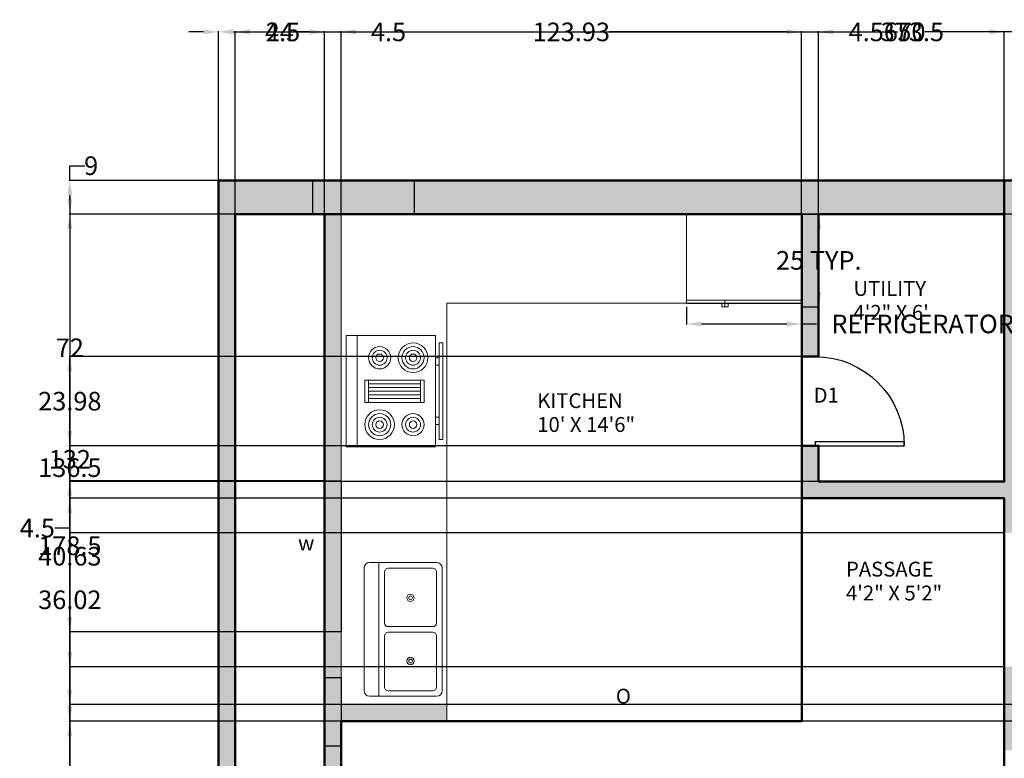
# Model space of a CAD drawing. Units: inches. Extents: x -12 to 887, y 330 to 874.
# Tile 3 of 9: x -12 to 253, y 675 to 874. Entities that reach past the tile are written whole.
import ezdxf

# ---------------------------------------------------------------- set-up
doc = ezdxf.new("R2010")
doc.units = ezdxf.units.IN
doc.header["$MEASUREMENT"] = 0
for name, color, linetype, lineweight in [('A-ANNO-DIMS', 2, 'Continuous', 18), ('A-ANNO-TEXT', 3, 'Continuous', 18), ('A-AREA-IDEN', 7, 'Continuous', 18), ('A-DOOR', 4, 'Continuous', 25), ('A-EQPM', 8, 'Continuous', 18), ('A-FLOR-FIXT', 8, 'Continuous', 18), ('A-GLAZ', 4, 'Continuous', 25), ('A-WALL', 7, 'Continuous', 50), ('A-WALL-PATT', 5, 'Continuous', 13)]:
    doc.layers.add(name, color=color, linetype=linetype, lineweight=lineweight)
doc.styles.get("Standard").update_dxf_attribs({"font": 'arial.ttf'})
doc.dimstyles.get("Standard").update_dxf_attribs({"dimtxt": 5, "dimasz": 4, "dimexe": 0.18, "dimexo": 0.0625, "dimgap": 0.09, "dimtad": 0, "dimtih": 1, "dimtoh": 1, "dimdec": 1, "dimzin": 0, "dimdsep": 46, "dimlunit": 4, "dimtxsty": 'Standard', "dimcen": 0.09, "dimadec": 0, "dimazin": 0, "dimtfac": 1, "dimtdec": 1, "dimtofl": 0, "dimtmove": 0, "dimatfit": 3, "dimfxl": 1, "dimtolj": 1, "dimtzin": 0, "dimarcsym": 0})

# ---------------------------------------------------------------- blocks, each defined once
blk = doc.blocks.new('Sink-double - 36 in top')
for p, q in [((-18, -4), (18, -4)), ((-0.75, -18.5), (-0.75, -6.5)), ((0.75, -6.5), (0.75, -18.5))]:
    blk.add_line(p, q)
for points in [[(-16.5, 0), (16.5, 0)], [(-18, -19.5), (-18, -1.5)], [(18, -1.5), (18, -19.5)], [(-16.5, -18.5), (-16.5, -6.5)], [(-15.5, -5.5), (-1.75, -5.5)], [(1.75, -5.5), (15.5, -5.5)], [(16.5, -6.5), (16.5, -18.5)], [(16.5, -21), (-16.5, -21)], [(-1.75, -19.5), (-15.5, -19.5)], [(15.5, -19.5), (1.75, -19.5)]]:
    blk.add_lwpolyline(points)
for centre, radius in [((-8.5, -12.5), 1), ((-8.5, -12.5), 0.5), ((8.5, -12.5), 1), ((8.5, -12.5), 0.5)]:
    blk.add_circle(centre, radius)
for centre, radius, start, end in [((-16.5, -1.5), 1.5, 90, 180), ((16.5, -1.5), 1.5, 0, 90), ((-15.5, -6.5), 1, 90, 180), ((-1.75, -6.5), 1, 0, 90), ((1.75, -6.5), 1, 90, 180), ((15.5, -6.5), 1, 0, 90), ((-15.5, -18.5), 1, 180, 270), ((-1.75, -18.5), 1, 270, 0), ((1.75, -18.5), 1, 180, 270), ((15.5, -18.5), 1, 270, 0), ((-16.5, -19.5), 1.5, 180, 270), ((16.5, -19.5), 1.5, 270, 0)]:
    blk.add_arc(centre, radius, start, end)
blk = doc.blocks.new('Range-Oven - 30 in top')
for p, q in [((0, -3), (30, -3)), ((12, -6), (18, -6)), ((13, -20), (13, -6)), ((14, -6), (14, -20)), ((15, -20), (15, -6)), ((16, -6), (16, -20)), ((17, -20), (17, -6)), ((18, -20), (12, -20)), ((6, -24), (6, -25)), ((8, -25), (8, -24)), ((22, -25), (22, -24)), ((24, -24), (24, -25))]:
    blk.add_line(p, q)
for points in [[(0, -24), (0, 0), (30, 0), (30, -24)], [(12, -21), (12, -5), (18, -5), (18, -21)], [(2, -26), (2, -25), (28, -25), (28, -26)]]:
    blk.add_lwpolyline(points, close=True)
for centre, radius in [((6, -9), 4), ((6, -9), 3), ((6, -9), 2), ((24, -9), 3), ((24, -9), 2), ((6, -9), 1), ((24, -9), 1), ((6, -18), 3), ((24, -18), 4), ((24, -18), 3), ((6, -18), 2), ((6, -18), 1), ((24, -18), 2), ((24, -18), 1)]:
    blk.add_circle(centre, radius)
blk = doc.blocks.new('Refrigerator-2 door - 36 in top')
for p, q in [((0, -26.999999), (36, -26.999999)), ((12, -26.999999), (12, -28.999999)), ((11, -27.999999), (11, -28.999999)), ((11, -28.999999), (13, -28.999999)), ((13, -28.999999), (13, -27.999999))]:
    blk.add_line(p, q)
blk.add_lwpolyline([(0, -27.999999), (0, 0), (36, 0), (36, -27.999999)], close=True)
blk = doc.blocks.new('*U5')
for p, q in [((0, 0), (0, -6)), ((40, 0), (40, -6))]:
    blk.add_line(p, q)
blk.add_lwpolyline([(0, 0), (0, 40), (1.75, 40), (1.75, 0)], close=True)
blk.add_arc((0, 0), 40, 0, 90)
blk = doc.blocks.new('*D28')
at = {"layer": 'A-ANNO-DIMS', "color": 0, "lineweight": -2, "transparency": 16777216}
for p, q in [((167.93, 796.66), (167.93, 791.9)), ((198.86, 796.66), (198.86, 791.9)), ((171.93, 792.08), (194.86, 792.08)), ((198.86, 792.08), (202.86, 792.08))]:
    blk.add_line(p, q, dxfattribs=at)
at = {"layer": 'A-ANNO-DIMS', "color": 0, "transparency": 16777216}
for points in [[(171.93, 792.75), (171.93, 791.42), (167.93, 792.08)], [(194.86, 792.75), (194.86, 791.42), (198.86, 792.08)]]:
    blk.add_solid(points, dxfattribs=at)
at = {"layer": 'Defpoints', "color": 0, "transparency": 16777216}
for p in [(167.93, 796.72), (198.86, 796.72), (198.86, 792.08)]:
    blk.add_point(p, dxfattribs=at)
at = {"layer": 'A-ANNO-DIMS', "color": 0, "transparency": 16777216, "insert": (243.71, 792.08), "char_height": 5, "attachment_point": 5}
blk.add_mtext('\\A1;REFRIGERATOR 31 TYP.', dxfattribs=at)
blk = doc.blocks.new('*D29')
at = {"layer": 'A-ANNO-DIMS', "color": 0, "lineweight": -2, "transparency": 16777216}
for p, q in [((198.92, 821.64), (203.68, 821.64)), ((203.5, 817.64), (203.5, 811.82)), ((203.5, 800.72), (203.5, 806.54)), ((198.92, 796.72), (203.68, 796.72))]:
    blk.add_line(p, q, dxfattribs=at)
at = {"layer": 'A-ANNO-DIMS', "color": 0, "transparency": 16777216}
for points in [[(202.83, 817.64), (204.17, 817.64), (203.5, 821.64)], [(202.83, 800.72), (204.17, 800.72), (203.5, 796.72)]]:
    blk.add_solid(points, dxfattribs=at)
at = {"layer": 'Defpoints', "color": 0, "transparency": 16777216}
for p in [(198.86, 821.64), (203.5, 821.64), (198.86, 796.72)]:
    blk.add_point(p, dxfattribs=at)
at = {"layer": 'A-ANNO-DIMS', "color": 0, "transparency": 16777216, "insert": (203.5, 809.18), "char_height": 5, "attachment_point": 5}
blk.add_mtext('\\A1;25 TYP.', dxfattribs=at)
blk = doc.blocks.new('*D38')
at = {"layer": 'A-ANNO-DIMS', "color": 0, "lineweight": -2, "transparency": 16777216}
for p, q in [((41.93, 830.72), (41.93, 870.84)), ((45.93, 870.66), (220.13, 870.66)), ((411.43, 870.66), (237.22, 870.66)), ((415.43, 830.72), (415.43, 870.84))]:
    blk.add_line(p, q, dxfattribs=at)
at = {"layer": 'A-ANNO-DIMS', "color": 0, "transparency": 16777216}
for points in [[(45.93, 871.33), (45.93, 869.99), (41.93, 870.66)], [(411.43, 871.33), (411.43, 869.99), (415.43, 870.66)]]:
    blk.add_solid(points, dxfattribs=at)
at = {"layer": 'Defpoints', "color": 0, "transparency": 16777216}
for p in [(415.43, 870.66), (41.93, 830.66), (415.43, 830.66)]:
    blk.add_point(p, dxfattribs=at)
at = {"layer": 'A-ANNO-DIMS', "color": 0, "transparency": 16777216, "insert": (228.68, 870.66), "char_height": 5, "attachment_point": 5}
blk.add_mtext('\\A1;373.5', dxfattribs=at)
blk = doc.blocks.new('*D39')
at = {"layer": 'A-ANNO-DIMS', "color": 0, "lineweight": -2, "transparency": 16777216}
for p, q in [((37.93, 870.66), (33.93, 870.66)), ((41.93, 830.72), (41.93, 870.84)), ((46.43, 821.72), (46.43, 870.84)), ((50.43, 870.66), (54.43, 870.66))]:
    blk.add_line(p, q, dxfattribs=at)
at = {"layer": 'A-ANNO-DIMS', "color": 0, "transparency": 16777216}
for points in [[(37.93, 871.33), (37.93, 869.99), (41.93, 870.66)], [(50.43, 871.33), (50.43, 869.99), (46.43, 870.66)]]:
    blk.add_solid(points, dxfattribs=at)
at = {"layer": 'Defpoints', "color": 0, "transparency": 16777216}
for p in [(46.43, 870.66), (41.93, 830.66), (46.43, 821.66)]:
    blk.add_point(p, dxfattribs=at)
at = {"layer": 'A-ANNO-DIMS', "color": 0, "transparency": 16777216, "insert": (59.19, 870.66), "char_height": 5, "attachment_point": 5}
blk.add_mtext('\\A1;4.5', dxfattribs=at)
blk = doc.blocks.new('*D40')
at = {"layer": 'A-ANNO-DIMS', "color": 0, "lineweight": -2, "transparency": 16777216}
for p, q in [((46.43, 821.72), (46.43, 870.84)), ((50.43, 870.66), (54.72, 870.66)), ((66.43, 870.66), (62.13, 870.66)), ((70.43, 821.72), (70.43, 870.84))]:
    blk.add_line(p, q, dxfattribs=at)
at = {"layer": 'A-ANNO-DIMS', "color": 0, "transparency": 16777216}
for points in [[(50.43, 871.33), (50.43, 869.99), (46.43, 870.66)], [(66.43, 871.33), (66.43, 869.99), (70.43, 870.66)]]:
    blk.add_solid(points, dxfattribs=at)
at = {"layer": 'Defpoints', "color": 0, "transparency": 16777216}
for p in [(70.43, 870.66), (46.43, 821.66), (70.43, 821.66)]:
    blk.add_point(p, dxfattribs=at)
at = {"layer": 'A-ANNO-DIMS', "color": 0, "transparency": 16777216, "insert": (58.43, 870.66), "char_height": 5, "attachment_point": 5}
blk.add_mtext('\\A1;24', dxfattribs=at)
blk = doc.blocks.new('*D41')
at = {"layer": 'A-ANNO-DIMS', "color": 0, "lineweight": -2, "transparency": 16777216}
for p, q in [((66.43, 870.66), (62.43, 870.66)), ((70.43, 821.72), (70.43, 870.84)), ((74.93, 821.72), (74.93, 870.84)), ((78.93, 870.66), (82.93, 870.66))]:
    blk.add_line(p, q, dxfattribs=at)
at = {"layer": 'A-ANNO-DIMS', "color": 0, "transparency": 16777216}
for points in [[(66.43, 871.33), (66.43, 869.99), (70.43, 870.66)], [(78.93, 871.33), (78.93, 869.99), (74.93, 870.66)]]:
    blk.add_solid(points, dxfattribs=at)
at = {"layer": 'Defpoints', "color": 0, "transparency": 16777216}
for p in [(74.93, 870.66), (70.43, 821.66), (74.93, 821.66)]:
    blk.add_point(p, dxfattribs=at)
at = {"layer": 'A-ANNO-DIMS', "color": 0, "transparency": 16777216, "insert": (87.69, 870.66), "char_height": 5, "attachment_point": 5}
blk.add_mtext('\\A1;4.5', dxfattribs=at)
blk = doc.blocks.new('*D42')
at = {"layer": 'A-ANNO-DIMS', "color": 0, "lineweight": -2, "transparency": 16777216}
for p, q in [((74.93, 821.72), (74.93, 870.84)), ((78.93, 870.66), (126.66, 870.66)), ((194.86, 870.66), (147.13, 870.66)), ((198.86, 821.7), (198.86, 870.84))]:
    blk.add_line(p, q, dxfattribs=at)
at = {"layer": 'A-ANNO-DIMS', "color": 0, "transparency": 16777216}
for points in [[(78.93, 871.33), (78.93, 869.99), (74.93, 870.66)], [(194.86, 871.33), (194.86, 869.99), (198.86, 870.66)]]:
    blk.add_solid(points, dxfattribs=at)
at = {"layer": 'Defpoints', "color": 0, "transparency": 16777216}
for p in [(198.86, 870.66), (74.93, 821.66), (198.86, 821.64)]:
    blk.add_point(p, dxfattribs=at)
at = {"layer": 'A-ANNO-DIMS', "color": 0, "transparency": 16777216, "insert": (136.89, 870.66), "char_height": 5, "attachment_point": 5}
blk.add_mtext('\\A1;123.93', dxfattribs=at)
blk = doc.blocks.new('*D43')
at = {"layer": 'A-ANNO-DIMS', "color": 0, "lineweight": -2, "transparency": 16777216}
for p, q in [((194.86, 870.66), (190.86, 870.66)), ((198.86, 821.7), (198.86, 870.84)), ((203.43, 821.72), (203.43, 870.84)), ((207.43, 870.66), (211.43, 870.66))]:
    blk.add_line(p, q, dxfattribs=at)
at = {"layer": 'A-ANNO-DIMS', "color": 0, "transparency": 16777216}
for points in [[(194.86, 871.33), (194.86, 869.99), (198.86, 870.66)], [(207.43, 871.33), (207.43, 869.99), (203.43, 870.66)]]:
    blk.add_solid(points, dxfattribs=at)
at = {"layer": 'Defpoints', "color": 0, "transparency": 16777216}
for p in [(203.43, 870.66), (198.86, 821.64), (203.43, 821.66)]:
    blk.add_point(p, dxfattribs=at)
at = {"layer": 'A-ANNO-DIMS', "color": 0, "transparency": 16777216, "insert": (220.05, 870.66), "char_height": 5, "attachment_point": 5}
blk.add_mtext('\\A1;4.567', dxfattribs=at)
blk = doc.blocks.new('*D44')
at = {"layer": 'A-ANNO-DIMS', "color": 0, "lineweight": -2, "transparency": 16777216}
for p, q in [((203.43, 821.72), (203.43, 870.84)), ((207.43, 870.66), (224.76, 870.66)), ((249.43, 870.66), (232.09, 870.66)), ((253.43, 821.72), (253.43, 870.84))]:
    blk.add_line(p, q, dxfattribs=at)
at = {"layer": 'A-ANNO-DIMS', "color": 0, "transparency": 16777216}
for points in [[(207.43, 871.33), (207.43, 869.99), (203.43, 870.66)], [(249.43, 871.33), (249.43, 869.99), (253.43, 870.66)]]:
    blk.add_solid(points, dxfattribs=at)
at = {"layer": 'Defpoints', "color": 0, "transparency": 16777216}
for p in [(253.43, 870.66), (203.43, 821.66), (253.43, 821.66)]:
    blk.add_point(p, dxfattribs=at)
at = {"layer": 'A-ANNO-DIMS', "color": 0, "transparency": 16777216, "insert": (228.43, 870.66), "char_height": 5, "attachment_point": 5}
blk.add_mtext('\\A1;50', dxfattribs=at)
blk = doc.blocks.new('*D45')
at = {"layer": 'A-ANNO-DIMS', "color": 0, "lineweight": -2, "transparency": 16777216}
for p, q in [((249.43, 870.66), (245.43, 870.66)), ((253.43, 821.72), (253.43, 870.84)), ((257.93, 821.72), (257.93, 870.84)), ((261.93, 870.66), (265.93, 870.66))]:
    blk.add_line(p, q, dxfattribs=at)
at = {"layer": 'A-ANNO-DIMS', "color": 0, "transparency": 16777216}
for points in [[(249.43, 871.33), (249.43, 869.99), (253.43, 870.66)], [(261.93, 871.33), (261.93, 869.99), (257.93, 870.66)]]:
    blk.add_solid(points, dxfattribs=at)
at = {"layer": 'Defpoints', "color": 0, "transparency": 16777216}
for p in [(257.93, 870.66), (253.43, 821.66), (257.93, 821.66)]:
    blk.add_point(p, dxfattribs=at)
at = {"layer": 'A-ANNO-DIMS', "color": 0, "transparency": 16777216, "insert": (270.69, 870.66), "char_height": 5, "attachment_point": 5}
blk.add_mtext('\\A1;4.5', dxfattribs=at)
blk = doc.blocks.new('*D53')
at = {"layer": 'A-ANNO-DIMS', "color": 0, "lineweight": -2, "transparency": 16777216}
for p, q in [((41.86, 830.66), (1.75, 830.66)), ((1.93, 826.66), (1.93, 604.54)), ((1.93, 377.16), (1.93, 599.28)), ((41.86, 373.16), (1.75, 373.16))]:
    blk.add_line(p, q, dxfattribs=at)
at = {"layer": 'A-ANNO-DIMS', "color": 0, "transparency": 16777216}
for points in [[(1.26, 826.66), (2.59, 826.66), (1.93, 830.66)], [(1.26, 377.16), (2.59, 377.16), (1.93, 373.16)]]:
    blk.add_solid(points, dxfattribs=at)
at = {"layer": 'Defpoints', "color": 0, "transparency": 16777216}
for p in [(1.93, 830.66), (41.93, 830.66), (41.93, 373.16)]:
    blk.add_point(p, dxfattribs=at)
at = {"layer": 'A-ANNO-DIMS', "color": 0, "transparency": 16777216, "insert": (1.93, 601.91), "char_height": 5, "attachment_point": 5}
blk.add_mtext('\\A1;457.5', dxfattribs=at)
blk = doc.blocks.new('*D57')
at = {"layer": 'A-ANNO-DIMS', "color": 0, "lineweight": -2, "transparency": 16777216}
for p, q in [((74.86, 685.16), (1.75, 685.16)), ((1.93, 681.16), (1.93, 628.55)), ((1.93, 570.66), (1.93, 623.27)), ((74.86, 566.66), (1.75, 566.66))]:
    blk.add_line(p, q, dxfattribs=at)
at = {"layer": 'A-ANNO-DIMS', "color": 0, "transparency": 16777216}
for points in [[(1.26, 681.16), (2.59, 681.16), (1.93, 685.16)], [(1.26, 570.66), (2.59, 570.66), (1.93, 566.66)]]:
    blk.add_solid(points, dxfattribs=at)
at = {"layer": 'Defpoints', "color": 0, "transparency": 16777216}
for p in [(1.93, 685.16), (74.93, 685.16), (74.93, 566.66)]:
    blk.add_point(p, dxfattribs=at)
at = {"layer": 'A-ANNO-DIMS', "color": 0, "transparency": 16777216, "insert": (1.93, 625.91), "char_height": 5, "attachment_point": 5}
blk.add_mtext('\\A1;118.5', dxfattribs=at)
blk = doc.blocks.new('*D58')
at = {"layer": 'A-ANNO-DIMS', "color": 0, "lineweight": -2, "transparency": 16777216}
for p, q in [((74.86, 821.66), (1.75, 821.66)), ((1.93, 817.66), (1.93, 756.06)), ((1.93, 689.16), (1.93, 750.77)), ((74.86, 685.16), (1.75, 685.16))]:
    blk.add_line(p, q, dxfattribs=at)
at = {"layer": 'A-ANNO-DIMS', "color": 0, "transparency": 16777216}
for points in [[(1.26, 817.66), (2.59, 817.66), (1.93, 821.66)], [(1.26, 689.16), (2.59, 689.16), (1.93, 685.16)]]:
    blk.add_solid(points, dxfattribs=at)
at = {"layer": 'Defpoints', "color": 0, "transparency": 16777216}
for p in [(1.93, 821.66), (74.93, 821.66), (74.93, 685.16)]:
    blk.add_point(p, dxfattribs=at)
at = {"layer": 'A-ANNO-DIMS', "color": 0, "transparency": 16777216, "insert": (1.93, 753.41), "char_height": 5, "attachment_point": 5}
blk.add_mtext('\\A1;136.5', dxfattribs=at)
blk = doc.blocks.new('*D59')
at = {"layer": 'A-ANNO-DIMS', "color": 0, "lineweight": -2, "transparency": 16777216}
for p, q in [((1.93, 830.66), (1.93, 834.66)), ((1.93, 834.66), (5.93, 834.66)), ((41.86, 830.66), (1.75, 830.66)), ((1.93, 825.66), (1.93, 826.66)), ((74.86, 821.66), (1.75, 821.66))]:
    blk.add_line(p, q, dxfattribs=at)
at = {"layer": 'A-ANNO-DIMS', "color": 0, "transparency": 16777216}
for points in [[(1.26, 826.66), (2.59, 826.66), (1.93, 830.66)], [(1.26, 825.66), (2.59, 825.66), (1.93, 821.66)]]:
    blk.add_solid(points, dxfattribs=at)
at = {"layer": 'Defpoints', "color": 0, "transparency": 16777216}
for p in [(1.93, 830.66), (41.93, 830.66), (74.93, 821.66)]:
    blk.add_point(p, dxfattribs=at)
at = {"layer": 'A-ANNO-DIMS', "color": 0, "transparency": 16777216, "insert": (7.66, 834.66), "char_height": 5, "attachment_point": 5}
blk.add_mtext('\\A1;9', dxfattribs=at)
blk = doc.blocks.new('*D69')
at = {"layer": 'A-ANNO-DIMS', "color": 0, "lineweight": -2, "transparency": 16777216}
for p, q in [((319.86, 685.16), (1.75, 685.16)), ((1.93, 681.16), (1.93, 660.79)), ((1.93, 635.16), (1.93, 655.53)), ((319.86, 631.16), (1.75, 631.16))]:
    blk.add_line(p, q, dxfattribs=at)
at = {"layer": 'A-ANNO-DIMS', "color": 0, "transparency": 16777216}
for points in [[(1.26, 681.16), (2.59, 681.16), (1.93, 685.16)], [(1.26, 635.16), (2.59, 635.16), (1.93, 631.16)]]:
    blk.add_solid(points, dxfattribs=at)
at = {"layer": 'Defpoints', "color": 0, "transparency": 16777216}
for p in [(1.93, 685.16), (319.93, 685.16), (319.93, 631.16)]:
    blk.add_point(p, dxfattribs=at)
at = {"layer": 'A-ANNO-DIMS', "color": 0, "transparency": 16777216, "insert": (1.93, 658.16), "char_height": 5, "attachment_point": 5}
blk.add_mtext('\\A1;54', dxfattribs=at)
blk = doc.blocks.new('*D72')
at = {"layer": 'A-ANNO-DIMS', "color": 0, "lineweight": -2, "transparency": 16777216}
for p, q in [((1.93, 753.66), (1.93, 757.66)), ((203.36, 749.66), (1.75, 749.66)), ((198.86, 745.16), (1.75, 745.16)), ((1.93, 741.16), (1.93, 737.16)), ((1.93, 737.16), (-2.07, 737.16))]:
    blk.add_line(p, q, dxfattribs=at)
at = {"layer": 'A-ANNO-DIMS', "color": 0, "transparency": 16777216}
for points in [[(1.26, 753.66), (2.59, 753.66), (1.93, 749.66)], [(1.26, 741.16), (2.59, 741.16), (1.93, 745.16)]]:
    blk.add_solid(points, dxfattribs=at)
at = {"layer": 'Defpoints', "color": 0, "transparency": 16777216}
for p in [(203.43, 749.66), (1.93, 745.16), (198.93, 745.16)]:
    blk.add_point(p, dxfattribs=at)
at = {"layer": 'A-ANNO-DIMS', "color": 0, "transparency": 16777216, "insert": (-6.83, 737.16), "char_height": 5, "attachment_point": 5}
blk.add_mtext('\\A1;4.5', dxfattribs=at)
blk = doc.blocks.new('*D73')
at = {"layer": 'A-ANNO-DIMS', "color": 0, "lineweight": -2, "transparency": 16777216}
for p, q in [((203.36, 821.66), (1.75, 821.66)), ((1.93, 817.66), (1.93, 788.26)), ((1.93, 753.66), (1.93, 783.06)), ((203.36, 749.66), (1.75, 749.66))]:
    blk.add_line(p, q, dxfattribs=at)
at = {"layer": 'A-ANNO-DIMS', "color": 0, "transparency": 16777216}
for points in [[(1.26, 817.66), (2.59, 817.66), (1.93, 821.66)], [(1.26, 753.66), (2.59, 753.66), (1.93, 749.66)]]:
    blk.add_solid(points, dxfattribs=at)
at = {"layer": 'Defpoints', "color": 0, "transparency": 16777216}
for p in [(1.93, 821.66), (203.43, 821.66), (203.43, 749.66)]:
    blk.add_point(p, dxfattribs=at)
at = {"layer": 'A-ANNO-DIMS', "color": 0, "transparency": 16777216, "insert": (1.93, 785.66), "char_height": 5, "attachment_point": 5}
blk.add_mtext('\\A1;72', dxfattribs=at)
blk = doc.blocks.new('*D78')
at = {"layer": 'A-ANNO-DIMS', "color": 0, "lineweight": -2, "transparency": 16777216}
for p, q in [((253.36, 735.87), (1.75, 735.87)), ((1.93, 731.87), (1.93, 720.51)), ((1.93, 703.85), (1.93, 715.22)), ((253.36, 699.85), (1.75, 699.85))]:
    blk.add_line(p, q, dxfattribs=at)
at = {"layer": 'A-ANNO-DIMS', "color": 0, "transparency": 16777216}
for points in [[(1.26, 731.87), (2.59, 731.87), (1.93, 735.87)], [(1.26, 703.85), (2.59, 703.85), (1.93, 699.85)]]:
    blk.add_solid(points, dxfattribs=at)
at = {"layer": 'Defpoints', "color": 0, "transparency": 16777216}
for p in [(253.43, 735.87), (1.93, 699.85), (253.43, 699.85)]:
    blk.add_point(p, dxfattribs=at)
at = {"layer": 'A-ANNO-DIMS', "color": 0, "transparency": 16777216, "insert": (1.93, 717.86), "char_height": 5, "attachment_point": 5}
blk.add_mtext('\\A1;36.02', dxfattribs=at)
blk = doc.blocks.new('*D79')
at = {"layer": 'A-ANNO-DIMS', "color": 0, "lineweight": -2, "transparency": 16777216}
for p, q in [((198.86, 783.29), (1.75, 783.29)), ((1.93, 779.29), (1.93, 773.94)), ((1.93, 763.31), (1.93, 768.65)), ((198.86, 759.31), (1.75, 759.31))]:
    blk.add_line(p, q, dxfattribs=at)
at = {"layer": 'A-ANNO-DIMS', "color": 0, "transparency": 16777216}
for points in [[(1.26, 779.29), (2.59, 779.29), (1.93, 783.29)], [(1.26, 763.31), (2.59, 763.31), (1.93, 759.31)]]:
    blk.add_solid(points, dxfattribs=at)
at = {"layer": 'Defpoints', "color": 0, "transparency": 16777216}
for p in [(198.93, 783.29), (1.93, 759.31), (198.93, 759.31)]:
    blk.add_point(p, dxfattribs=at)
at = {"layer": 'A-ANNO-DIMS', "color": 0, "transparency": 16777216, "insert": (1.93, 771.3), "char_height": 5, "attachment_point": 5}
blk.add_mtext('\\A1;23.98', dxfattribs=at)
blk = doc.blocks.new('*D81')
at = {"layer": 'A-ANNO-DIMS', "color": 0, "lineweight": -2, "transparency": 16777216}
for p, q in [((70.36, 749.9), (1.75, 749.9)), ((1.93, 745.9), (1.93, 732.22)), ((1.93, 713.26), (1.93, 726.93)), ((70.36, 709.26), (1.75, 709.26))]:
    blk.add_line(p, q, dxfattribs=at)
at = {"layer": 'A-ANNO-DIMS', "color": 0, "transparency": 16777216}
for points in [[(1.26, 745.9), (2.59, 745.9), (1.93, 749.9)], [(1.26, 713.26), (2.59, 713.26), (1.93, 709.26)]]:
    blk.add_solid(points, dxfattribs=at)
at = {"layer": 'Defpoints', "color": 0, "transparency": 16777216}
for p in [(70.43, 749.9), (1.93, 709.26), (70.43, 709.26)]:
    blk.add_point(p, dxfattribs=at)
at = {"layer": 'A-ANNO-DIMS', "color": 0, "transparency": 16777216, "insert": (1.93, 729.58), "char_height": 5, "attachment_point": 5}
blk.add_mtext('\\A1;40.63', dxfattribs=at)
blk = doc.blocks.new('*D102')
at = {"layer": 'A-ANNO-DIMS', "color": 0, "lineweight": -2, "transparency": 16777216}
for p, q in [((493.01, 821.66), (1.75, 821.66)), ((1.93, 817.66), (1.93, 735.05)), ((1.93, 647.16), (1.93, 729.77)), ((493.01, 643.16), (1.75, 643.16))]:
    blk.add_line(p, q, dxfattribs=at)
at = {"layer": 'A-ANNO-DIMS', "color": 0, "transparency": 16777216}
for points in [[(1.26, 817.66), (2.59, 817.66), (1.93, 821.66)], [(1.26, 647.16), (2.59, 647.16), (1.93, 643.16)]]:
    blk.add_solid(points, dxfattribs=at)
at = {"layer": 'Defpoints', "color": 0, "transparency": 16777216}
for p in [(1.93, 821.66), (493.07, 821.66), (493.07, 643.16)]:
    blk.add_point(p, dxfattribs=at)
at = {"layer": 'A-ANNO-DIMS', "color": 0, "transparency": 16777216, "insert": (1.93, 732.41), "char_height": 5, "attachment_point": 5}
blk.add_mtext('\\A1;178.5', dxfattribs=at)
blk = doc.blocks.new('*D103')
at = {"layer": 'A-ANNO-DIMS', "color": 0, "lineweight": -2, "transparency": 16777216}
for p, q in [((1.93, 830.66), (1.93, 834.66)), ((1.93, 834.66), (5.93, 834.66)), ((460.01, 830.66), (1.75, 830.66)), ((1.93, 825.66), (1.93, 826.66)), ((493.01, 821.66), (1.75, 821.66))]:
    blk.add_line(p, q, dxfattribs=at)
at = {"layer": 'A-ANNO-DIMS', "color": 0, "transparency": 16777216}
for points in [[(1.26, 826.66), (2.59, 826.66), (1.93, 830.66)], [(1.26, 825.66), (2.59, 825.66), (1.93, 821.66)]]:
    blk.add_solid(points, dxfattribs=at)
at = {"layer": 'Defpoints', "color": 0, "transparency": 16777216}
for p in [(1.93, 830.66), (460.07, 830.66), (493.07, 821.66)]:
    blk.add_point(p, dxfattribs=at)
at = {"layer": 'A-ANNO-DIMS', "color": 0, "transparency": 16777216, "insert": (7.66, 834.66), "char_height": 5, "attachment_point": 5}
blk.add_mtext('\\A1;9', dxfattribs=at)
blk = doc.blocks.new('*D112')
at = {"layer": 'A-ANNO-DIMS', "color": 0, "lineweight": -2, "transparency": 16777216}
for p, q in [((676.01, 821.66), (1.75, 821.66)), ((1.93, 817.66), (1.93, 758.31)), ((1.93, 693.66), (1.93, 753.02)), ((676.01, 689.66), (1.75, 689.66))]:
    blk.add_line(p, q, dxfattribs=at)
at = {"layer": 'A-ANNO-DIMS', "color": 0, "transparency": 16777216}
for points in [[(1.26, 817.66), (2.59, 817.66), (1.93, 821.66)], [(1.26, 693.66), (2.59, 693.66), (1.93, 689.66)]]:
    blk.add_solid(points, dxfattribs=at)
at = {"layer": 'Defpoints', "color": 0, "transparency": 16777216}
for p in [(1.93, 821.66), (676.07, 821.66), (676.07, 689.66)]:
    blk.add_point(p, dxfattribs=at)
at = {"layer": 'A-ANNO-DIMS', "color": 0, "transparency": 16777216, "insert": (1.93, 755.66), "char_height": 5, "attachment_point": 5}
blk.add_mtext('\\A1;132', dxfattribs=at)

msp = doc.modelspace()

# ---------------------------------------------------------------- hatches: boundary and pattern name
at = {"layer": 'A-WALL-PATT'}
h = msp.add_hatch(color=256, dxfattribs=at)
h.dxf.hatch_style = 1
h.paths.add_polyline_path([(253.4263, 830.6611), (94.575, 830.6611), (94.575, 821.6611), (198.9263, 821.6611), (198.9263, 783.3094), (203.4263, 783.3094), (203.4263, 821.6611), (253.4263, 821.6611)], flags=17)
h.paths.add_polyline_path([(415.4263, 830.6611), (392.9263, 830.6611), (392.9263, 821.6611), (410.9263, 821.6611), (410.9263, 701.6611), (410.9263, 382.1611), (392.9263, 382.1611), (392.9263, 450.1611), (383.9263, 450.1611), (383.9263, 382.1611), (253.4263, 382.1611), (46.4263, 382.1611), (46.4263, 821.6611), (67.3199, 821.6611), (67.3199, 830.6611), (41.9263, 830.6611), (41.9263, 373.1611), (253.4263, 373.1611), (415.4263, 373.1611)])
h.paths.add_polyline_path([(364.023, 830.6611), (288.8031, 830.6611), (288.8031, 821.6611), (364.023, 821.6611)], flags=17)
h.paths.add_polyline_path([(257.9263, 821.6611), (253.4263, 821.6611), (253.4263, 749.6611), (203.4263, 749.6611), (203.4263, 759.3094), (198.9263, 759.3094), (198.9263, 745.1611), (253.4263, 745.1611), (253.4263, 735.8547), (257.9263, 735.8547)], flags=17)
h.paths.add_polyline_path([(257.9263, 653.338), (257.0311, 653.338), (253.4263, 653.338), (253.4263, 579.1607), (257.9263, 579.1607)], flags=17)
h.paths.add_polyline_path([(323.9263, 685.1611), (328.2749, 685.1611), (328.2749, 689.6611), (257.9263, 689.6611), (257.9263, 685.1611), (319.9263, 685.1611), (319.9263, 631.1611), (257.9263, 631.1611), (257.9263, 626.6611), (319.9263, 626.6611), (319.9263, 566.6611), (286.6409, 566.6611, -0.00931598), (286.6576, 565.7658), (286.6576, 562.1611), (383.9263, 562.1611), (383.9263, 566.6611), (323.9263, 566.6611)], flags=17)
h.paths.add_polyline_path([(142.5107, 566.6611), (135.5357, 566.6611), (135.5357, 562.1611), (142.5107, 562.1611)], flags=17)
h.paths.add_polyline_path([(253.4263, 566.6611), (229.0035, 566.6611), (229.0035, 562.1611), (253.4263, 562.1611)], flags=17)
h.paths.add_polyline_path([(262.6261, 566.6611), (257.9263, 566.6611), (257.9263, 562.1611), (262.6261, 562.1611)], flags=17)
h.paths.add_polyline_path([(392.9263, 553.5254), (383.9263, 553.5254), (383.9263, 454.1611), (392.9263, 454.1611)], flags=17)
h.paths.add_polyline_path([(353.8031, 418.1611), (247.9263, 418.1611), (247.9263, 414.1611), (353.8031, 414.1611)], flags=17)
h.paths.add_polyline_path([(374.959, 454.1611), (272.0195, 454.1611), (272.0195, 450.1611), (374.959, 450.1611)], flags=17)
h.paths.add_polyline_path([(254.2006, 454.1611), (247.9263, 454.1611), (247.9263, 450.1611), (254.2006, 450.1611)], flags=17)
h = msp.add_hatch(color=256, dxfattribs=at)
h.dxf.hatch_style = 1
h.paths.add_polyline_path([(94.575, 830.6611), (67.3199, 830.6611), (67.3199, 821.6611), (70.4263, 821.6611), (79.4263, 821.6611), (94.575, 821.6611)])
h.paths.add_polyline_path([(288.8031, 830.6611), (257.9263, 830.6611), (253.4263, 830.6611), (253.4263, 821.6611), (288.8031, 821.6611)])
h.paths.add_polyline_path([(74.9263, 696.9265), (70.4263, 696.9265), (70.4263, 678.4656), (74.9263, 678.4656)])
h.paths.add_polyline_path([(74.9263, 584.8756), (70.4263, 584.8756), (70.4263, 562.1611), (74.9263, 562.1611)])
h.paths.add_polyline_path([(135.5357, 566.6611), (122.6994, 566.6611), (122.6994, 562.1611), (135.5357, 562.1611)])
h.paths.add_polyline_path([(257.9263, 579.1607), (253.4263, 579.1607), (253.4263, 562.1611), (257.9263, 562.1611)])
h.paths.add_polyline_path([(272.0195, 454.1611), (254.2006, 454.1611), (254.2006, 450.1611), (272.0195, 450.1611)])
h.paths.add_polyline_path([(392.9263, 454.1611), (374.959, 454.1611), (374.959, 450.1611), (383.9263, 450.1611), (392.9263, 450.1611)])
h.paths.add_polyline_path([(493.0683, 466.4171), (488.5683, 466.4171), (488.5683, 450.1611), (493.0683, 450.1611)])
h.paths.add_polyline_path([(568.6302, 454.1611), (555.938, 454.1611), (555.938, 450.1611), (568.6302, 450.1611)])
h.paths.add_polyline_path([(493.0683, 594.9471), (488.5683, 594.9471), (488.5683, 569.5862), (493.0683, 569.5862)])
h.paths.add_polyline_path([(690.1615, 454.1611), (672.3426, 454.1611), (672.3426, 450.1611), (690.1615, 450.1611)])
h.paths.add_polyline_path([(811.0683, 454.1611), (793.101, 454.1611), (793.101, 450.1611), (802.0683, 450.1611), (811.0683, 450.1611)])
h.paths.add_polyline_path([(811.0683, 578.3606), (802.0683, 578.3606), (802.0683, 566.6611), (802.0683, 553.5254), (811.0683, 553.5254)])
h.paths.add_polyline_path([(811.0683, 701.6611), (802.0683, 701.6611), (802.0683, 689.9616), (802.0683, 676.8259), (811.0683, 676.8259)])
h.paths.add_polyline_path([(811.0683, 830.6611), (782.165, 830.6611), (782.165, 821.6611), (802.0683, 821.6611), (811.0683, 821.6611)])
h.paths.add_polyline_path([(706.9451, 830.6611), (671.5683, 830.6611), (671.5683, 821.6611), (706.9451, 821.6611)])
h.paths.add_polyline_path([(512.717, 830.6611), (485.4619, 830.6611), (485.4619, 821.6611), (488.5683, 821.6611), (512.717, 821.6611)])
h.paths.add_polyline_path([(392.9263, 697.8668), (383.9263, 697.8668), (383.9263, 689.6611), (383.9263, 676.5034), (392.9263, 676.5034)])
h.paths.add_polyline_path([(392.9263, 830.6611), (364.023, 830.6611), (364.023, 821.7357), (392.9263, 821.7357)])
h.paths.add_polyline_path([(392.9263, 619.0434), (383.9263, 619.0434), (383.9263, 588.7499), (392.9263, 588.7499)])
h.paths.add_polyline_path([(392.9263, 578.3606), (383.9263, 578.3606), (383.9263, 566.6611), (383.9263, 553.5254), (392.9263, 553.5254)])
h.paths.add_polyline_path([(257.9263, 699.8547), (253.4263, 699.8547), (253.4263, 697.1611), (253.4263, 677.338), (257.9263, 677.338)])
h.paths.add_polyline_path([(493.0683, 714.3785), (488.5683, 714.3785), (488.5683, 689.6611), (493.0683, 689.6611)])
h.paths.add_polyline_path([(74.9263, 491.4191), (70.4263, 491.4191), (70.4263, 480.7097), (74.9263, 480.7097)])
h = msp.add_hatch(color=256, dxfattribs=at)
h.dxf.hatch_style = 1
h.paths.add_polyline_path([(86.6469, 566.6611), (74.9263, 566.6611), (74.9263, 562.1611), (86.6469, 562.1611)])
h.paths.add_polyline_path([(74.9263, 599.271), (70.4263, 599.271), (70.4263, 584.8756), (74.9263, 584.8756)])
h.paths.add_polyline_path([(74.9263, 678.4656), (70.4263, 678.4656), (70.4263, 671.2153), (74.9263, 671.2153)])
h.paths.add_polyline_path([(74.9263, 709.2627), (70.4263, 709.2627), (70.4263, 696.9265), (74.9263, 696.9265)])
h.paths.add_polyline_path([(74.9263, 821.6611), (70.4263, 821.6611), (70.4263, 749.8953), (74.9263, 749.8953)])
h.paths.add_polyline_path([(383.9263, 689.6611), (352.3064, 689.6611), (352.3064, 686.0564, -0.00931598), (352.2897, 685.1611), (383.9263, 685.1611)])
h.paths.add_polyline_path([(392.9263, 706.6608), (383.9263, 706.6608), (383.9263, 701.6611), (383.9263, 697.8668), (392.9263, 697.8668)])
h.paths.add_polyline_path([(392.9263, 821.7357), (383.9263, 821.7357), (383.9263, 751.0224), (383.9263, 742.7561), (392.9263, 742.7561)])
h.paths.add_polyline_path([(392.9263, 676.5034), (383.9263, 676.5034), (383.9263, 619.0434), (392.9263, 619.0434)])
h.paths.add_polyline_path([(392.9263, 588.7499), (383.9263, 588.7499), (383.9263, 578.3606), (392.9263, 578.3606)])
h = msp.add_hatch(color=256, dxfattribs=at)
h.dxf.hatch_style = 1
h.paths.add_polyline_path([(74.9263, 749.8953), (70.4263, 749.8953), (70.4263, 709.2627), (74.9263, 709.2627)])
h.paths.add_polyline_path([(74.9263, 671.2153), (70.4263, 671.2153), (70.4263, 599.271), (74.9263, 599.271)])
h.paths.add_polyline_path([(229.0035, 566.6611), (142.5107, 566.6611), (142.5107, 562.1611), (229.0035, 562.1611)])
h.paths.add_polyline_path([(392.9263, 742.7561), (383.9263, 742.7561), (383.9263, 706.6608), (392.9263, 706.6608)])
h.paths.add_polyline_path([(656.7304, 454.1611), (582.6585, 454.1611), (582.6585, 450.1611), (656.7304, 450.1611)])
h.paths.add_polyline_path([(493.0683, 557.2595), (488.5683, 557.2595), (488.5683, 492.3446), (493.0683, 492.3446)])
h.paths.add_polyline_path([(493.0683, 781.3634), (488.5683, 781.3634), (488.5683, 728.8273), (493.0683, 728.8273)])
h.paths.add_polyline_path([(811.0683, 756.0738), (802.0683, 756.0738), (802.0683, 707.8935), (811.0683, 707.8935)])
h = msp.add_hatch(color=256, dxfattribs=at)
h.dxf.hatch_style = 1
h.paths.add_polyline_path([(103.4263, 689.6611), (74.9263, 689.6611), (74.9263, 685.1611), (103.4263, 685.1611)])

# ---------------------------------------------------------------- linework, layer by layer
at = {"layer": 'A-FLOR-FIXT'}
for points in [[(74.9263, 821.6611), (74.9263, 689.6611), (103.4263, 689.6611)], [(103.4263, 685.1611), (103.4263, 797.6611), (198.9263, 797.6611)]]:
    msp.add_lwpolyline(points, dxfattribs=at)
at = {"layer": 'A-GLAZ'}
for points in [[(67.3199, 830.6611), (94.575, 830.6611), (94.575, 821.6611), (67.3199, 821.6611)], [(74.9263, 709.2627), (70.4263, 709.2627), (70.4263, 749.8953), (74.9263, 749.8953)], [(74.9263, 678.4656), (70.4263, 678.4656), (70.4263, 696.9265), (74.9263, 696.9265)]]:
    msp.add_lwpolyline(points, close=True, dxfattribs=at)
at = {"layer": 'A-WALL'}
msp.add_line((70.4263, 821.6611), (70.4263, 566.6611), dxfattribs=at)
msp.add_lwpolyline([(41.9263, 830.6611), (253.4263, 830.6611), (257.9263, 830.6611), (415.4263, 830.6611), (415.4263, 373.1611), (253.4263, 373.1611), (41.9263, 373.1611)], close=True, dxfattribs=at)
for points in [[(198.9263, 759.3094), (203.4263, 759.3094), (203.4263, 749.6611), (253.4263, 749.6611), (253.4263, 830.6611)], [(247.9263, 450.1611), (383.9263, 450.1611), (383.9263, 382.1611), (253.4263, 382.1611), (46.4263, 382.1611), (46.4263, 821.6611), (70.4263, 821.6611), (79.4263, 821.6611), (198.9263, 821.6611), (198.9263, 745.1611)], [(253.4263, 821.6611), (203.4263, 821.6611), (203.4263, 783.3094), (198.9263, 783.3094)], [(86.6469, 562.1611), (86.6469, 566.6611), (74.9263, 566.6611), (74.9263, 685.1611), (198.9263, 685.1611), (198.9263, 745.1611), (253.4263, 745.1611), (253.4263, 697.1611), (253.4263, 562.1611), (122.6469, 562.1611)]]:
    msp.add_lwpolyline(points, dxfattribs=at)

# ---------------------------------------------------------------- block references
at = {"layer": 'A-DOOR', "xscale": -0.5994880856815563, "yscale": 0.5994880856815563, "zscale": 0.5994880856815563, "rotation": 270}
msp.add_blockref('*U5', (202.5233, 759.3094), dxfattribs=at)
at = {"layer": 'A-EQPM', "xscale": 0.8591090410497297, "yscale": 0.8591090410497297, "zscale": 0.8591090410497297}
msp.add_blockref('Refrigerator-2 door - 36 in top', (167.9317, 821.6375), dxfattribs=at)
at = {"layer": 'A-EQPM', "rotation": 90}
msp.add_blockref('Range-Oven - 30 in top', (76.301, 758.9824), dxfattribs=at)
at = {"layer": 'A-FLOR-FIXT', "rotation": 90}
msp.add_blockref('Sink-double - 36 in top', (81.1197, 709.8814), dxfattribs=at)

# ---------------------------------------------------------------- texts
at = {"layer": 'A-ANNO-TEXT'}
for s, p in [('D1', (202.1037, 770.9029)), ('w', (63.348, 731.1332)), ('O ', (148.8823, 689.9293))]:
    msp.add_text(s, height=4, dxfattribs=at).set_placement(p)
at = {"layer": 'A-AREA-IDEN'}
for s, p in [('UTILITY', (212.8329, 799.615)), ('4\'2" X 6\'', (212.8329, 793.1894)), ('KITCHEN', (127.7248, 769.4457)), ('10\' X 14\'6"', (127.7248, 763.02)), ('PASSAGE', (210.8154, 724.1037)), ('4\'2" X 5\'2"', (210.8154, 717.6781))]:
    msp.add_text(s, height=4, dxfattribs=at).set_placement(p)

# ---------------------------------------------------------------- dimensions: what is measured, and where the dimension line sits
at = {"layer": 'A-ANNO-DIMS'}
for base, p1, p2, override, picture, middle in [((46.4263, 870.6611), (41.9263, 830.6611), (46.4263, 821.6611), {"dimdec": 1, "dimlfac": 1, "dimrnd": 0, "dimzin": 0, "dimdsep": 46, "dimlunit": 2}, '*D39', (59.1872, 870.6611)), ((415.4263, 870.6611), (41.9263, 830.6611), (415.4263, 830.6611), {"dimdec": 1, "dimlfac": 1, "dimrnd": 0, "dimzin": 0, "dimdsep": 46, "dimlunit": 2}, '*D38', (228.6763, 870.6611)), ((70.4263, 870.6611), (46.4263, 821.6611), (70.4263, 821.6611), {"dimdec": 0, "dimlfac": 1, "dimrnd": 0, "dimzin": 0, "dimdsep": 46, "dimlunit": 2}, '*D40', (58.4263, 870.6611)), ((74.9263, 870.6611), (70.4263, 821.6611), (74.9263, 821.6611), {"dimdec": 1, "dimlfac": 1, "dimrnd": 0, "dimzin": 0, "dimdsep": 46, "dimlunit": 2}, '*D41', (87.6872, 870.6611)), ((198.8596, 870.6611), (74.9263, 821.6611), (198.8596, 821.6375), {"dimdec": 2, "dimlfac": 1, "dimrnd": 0, "dimzin": 0, "dimdsep": 46, "dimlunit": 2}, '*D42', (136.893, 870.6611)), ((203.4263, 870.6611), (198.8596, 821.6375), (203.4263, 821.6611), {"dimdec": 3, "dimlfac": 1, "dimrnd": 0, "dimzin": 0, "dimdsep": 46, "dimlunit": 2}, '*D43', (220.0532, 870.6611)), ((253.4263, 870.6611), (203.4263, 821.6611), (253.4263, 821.6611), {"dimdec": 0, "dimlfac": 1, "dimrnd": 0, "dimzin": 0, "dimdsep": 46, "dimlunit": 2}, '*D44', (228.4263, 870.6611)), ((257.9263, 870.6611), (253.4263, 821.6611), (257.9263, 821.6611), {"dimdec": 1, "dimlfac": 1, "dimrnd": 0, "dimzin": 0, "dimdsep": 46, "dimlunit": 2}, '*D45', (270.6872, 870.6611))]:
    dim = msp.add_linear_dim(base=base, p1=p1, p2=p2, dimstyle='Standard', override=override, dxfattribs=at)
    dim.commit()
    dim.dimension.update_dxf_attribs({"geometry": picture, "text_midpoint": middle})
for base, p1, p2, override, picture, middle in [((1.9263, 830.6611), (74.9263, 821.6611), (41.9263, 830.6611), {"dimdec": 0, "dimlfac": 1, "dimrnd": 0, "dimzin": 0, "dimdsep": 46, "dimlunit": 2}, '*D59', (7.6603, 834.6611)), ((1.9263, 830.6611), (493.0683, 821.6611), (460.0683, 830.6611), {"dimdec": 0, "dimlfac": 1, "dimrnd": 0, "dimzin": 0, "dimdsep": 46, "dimlunit": 2}, '*D103', (7.6603, 834.6611)), ((1.9263, 830.6611), (41.9263, 373.1611), (41.9263, 830.6611), {"dimdec": 1, "dimlfac": 1, "dimrnd": 0, "dimzin": 0, "dimdsep": 46, "dimlunit": 2}, '*D53', (1.9263, 601.9111)), ((1.9263, 821.6611), (74.9263, 685.1611), (74.9263, 821.6611), {"dimdec": 1, "dimlfac": 1, "dimrnd": 0, "dimzin": 0, "dimdsep": 46, "dimlunit": 2}, '*D58', (1.9263, 753.4111)), ((1.9263, 821.6611), (493.0683, 643.1611), (493.0683, 821.6611), {"dimdec": 1, "dimlfac": 1, "dimrnd": 0, "dimzin": 0, "dimdsep": 46, "dimlunit": 2}, '*D102', (1.9263, 732.4111)), ((1.9263, 821.6611), (676.0683, 689.6611), (676.0683, 821.6611), {"dimdec": 0, "dimlfac": 1, "dimrnd": 0, "dimzin": 0, "dimdsep": 46, "dimlunit": 2}, '*D112', (1.9263, 755.6611)), ((1.9263, 821.6611), (203.4263, 749.6611), (203.4263, 821.6611), {"dimdec": 0, "dimlfac": 1, "dimrnd": 0, "dimzin": 0, "dimdsep": 46, "dimlunit": 2}, '*D73', (1.9263, 785.6611)), ((1.9263, 759.3094), (198.9263, 783.289), (198.9263, 759.3094), {"dimdec": 2, "dimlfac": 1, "dimrnd": 0, "dimzin": 0, "dimdsep": 46, "dimlunit": 2}, '*D79', (1.9263, 771.2992)), ((1.9263, 745.1611), (203.4263, 749.6611), (198.9263, 745.1611), {"dimdec": 1, "dimlfac": 1, "dimrnd": 0, "dimzin": 0, "dimdsep": 46, "dimlunit": 2}, '*D72', (-6.8345, 737.1611)), ((1.9263, 709.2627), (70.4263, 749.8953), (70.4263, 709.2627), {"dimdec": 2, "dimlfac": 1, "dimrnd": 0, "dimzin": 0, "dimdsep": 46, "dimlunit": 2}, '*D81', (1.9263, 729.579)), ((1.9263, 699.8547), (253.4263, 735.8743), (253.4263, 699.8547), {"dimdec": 2, "dimlfac": 1, "dimrnd": 0, "dimzin": 0, "dimdsep": 46, "dimlunit": 2}, '*D78', (1.9263, 717.8645)), ((1.9263, 685.1611), (74.9263, 566.6611), (74.9263, 685.1611), {"dimdec": 1, "dimlfac": 1, "dimrnd": 0, "dimzin": 0, "dimdsep": 46, "dimlunit": 2}, '*D57', (1.9263, 625.9111)), ((1.9263, 685.1611), (319.9263, 631.1611), (319.9263, 685.1611), {"dimdec": 0, "dimlfac": 1, "dimrnd": 0, "dimzin": 0, "dimdsep": 46, "dimlunit": 2}, '*D69', (1.9263, 658.1611))]:
    dim = msp.add_linear_dim(base=base, p1=p1, p2=p2, angle=90, dimstyle='Standard', override=override, dxfattribs=at)
    dim.commit()
    dim.dimension.update_dxf_attribs({"geometry": picture, "text_midpoint": middle})
dim = msp.add_linear_dim(base=(203.4988, 821.6375), p1=(198.8596, 796.7233), p2=(198.8596, 821.6375), angle=90, text='<> TYP.', dimstyle='Standard', override={"dimdec": 0, "dimrnd": 0, "dimzin": 0, "dimlunit": 2}, dxfattribs=at)
dim.commit()
dim.dimension.update_dxf_attribs({"geometry": '*D29', "text_midpoint": (203.4988, 809.1804)})
dim = msp.add_linear_dim(base=(198.8596, 792.0842), p1=(167.9317, 796.7233), p2=(198.8596, 796.7233), text='REFRIGERATOR <> TYP.', dimstyle='Standard', override={"dimdec": 0, "dimrnd": 0, "dimzin": 0, "dimlunit": 2}, dxfattribs=at)
dim.commit()
dim.dimension.update_dxf_attribs({"geometry": '*D28', "text_midpoint": (243.7068, 792.0842)})

doc.saveas('drawing.dxf')
